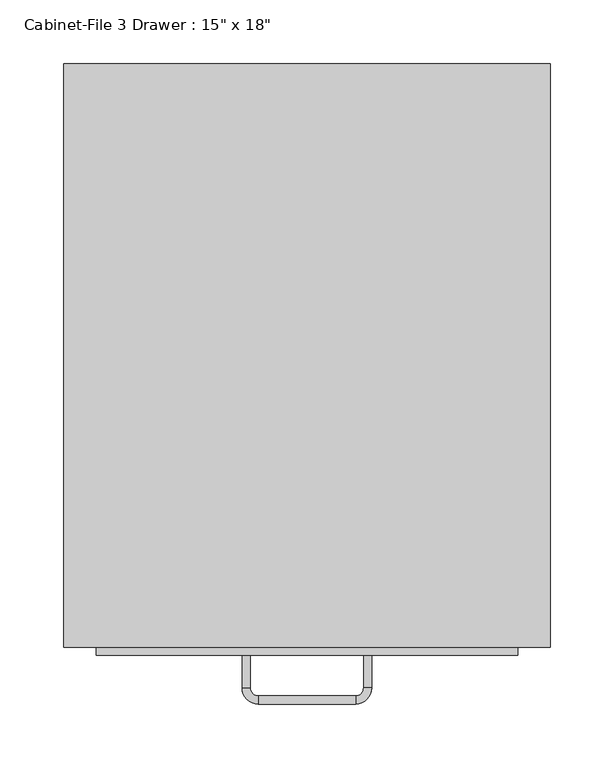
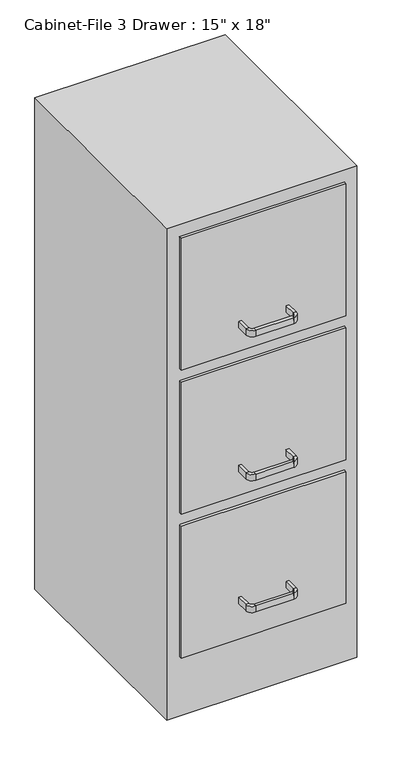
"""IFC4 building model written with IfcOpenShell, lengths in millimetres: furniture geometry."""

from ifc_helpers import new_model, si_unit, frame, origin, origin_with_axes, place, context, project, spatial, polyline, circle_curve, outline, extrude, source, transform, mapped, element, save
from ifc_brep_helpers import plane_surface, cylinder_surface, revolved_surface, advanced_brep


def furniture_552c1472(model_context):
    return source(origin(), model_context, "Body", "SolidModel", [
        extrude(outline(polyline([(62.603553, 86.4656999), (62.603553, -370.7343001), (-318.396447, -370.7343001), (-318.396447, 86.4656999), (62.603553, 86.4656999)])), origin_with_axes(), (0.0, 0.0, 1.0), 1041.4),
        extrude(outline(polyline([(37.203553, -377.0843001), (-292.996447, -377.0843001), (-292.996447, -370.7343001), (37.203553, -370.7343001), (37.203553, -377.0843001)])), frame((0.0, 0.0, 736.6), z_axis=(0.0, 0.0, 1.0), x_axis=(1.0, 0.0, 0.0)), (0.0, 0.0, 1.0), 279.4),
        extrude(outline(polyline([(37.203553, -377.0843001), (-292.996447, -377.0843001), (-292.996447, -370.7343001), (37.203553, -370.7343001), (37.203553, -377.0843001)])), frame((0.0, 0.0, 431.8), z_axis=(0.0, 0.0, 1.0), x_axis=(1.0, 0.0, 0.0)), (0.0, 0.0, 1.0), 279.4),
        extrude(outline(polyline([(37.203553, -377.0843001), (-292.996447, -377.0843001), (-292.996447, -370.7343001), (37.203553, -370.7343001), (37.203553, -377.0843001)])), frame((0.0, 0.0, 127.0), z_axis=(0.0, 0.0, 1.0), x_axis=(1.0, 0.0, 0.0)), (0.0, 0.0, 1.0), 279.4),
        advanced_brep(
        [(-172.346447, -377.0843001, 203.2), (-178.696447, -377.0843001, 203.2), (-178.696447, -377.0843001, 215.9), (-172.346447, -377.0843001, 215.9), (-172.346447, -402.4843001, 203.2), (-178.696447, -402.4843001, 203.2), (-178.696447, -402.4843001, 215.9), (-172.346447, -402.4843001, 215.9), (-165.996447, -415.1843001, 203.2), (-165.996447, -408.8343001, 203.2), (-165.996447, -415.1843001, 215.9), (-165.996447, -408.8343001, 215.9), (-89.796447, -408.8343001, 203.2), (-89.796447, -415.1843001, 203.2), (-89.796447, -415.1843001, 215.9), (-89.796447, -408.8343001, 215.9), (-77.096447, -402.4843001, 203.2), (-83.446447, -402.4843001, 203.2), (-77.096447, -402.4843001, 215.9), (-83.446447, -402.4843001, 215.9), (-83.446447, -377.0843001, 203.2), (-83.446447, -377.0843001, 215.9), (-77.096447, -377.0843001, 215.9), (-77.096447, -377.0843001, 203.2)],
        [
            (0, 1),
            (1, 2),
            (2, 3),
            (3, 0),
            (0, 4),
            (4, 5),
            (5, 1),
            (5, 6),
            (6, 2),
            (6, 7),
            (7, 3),
            (7, 4),
            (8, 5, circle_curve(frame((-165.996447, -402.4843001, 203.2), z_axis=(0.0, 0.0, -1.0), x_axis=(-1.0, 0.0, 0.0)), 12.7)),
            (4, 9, circle_curve(frame((-165.996447, -402.4843001, 203.2), z_axis=(0.0, 0.0, 1.0), x_axis=(-1.0, 0.0, 0.0)), 6.35)),
            (9, 8),
            (10, 6, circle_curve(frame((-165.996447, -402.4843001, 215.9), z_axis=(0.0, 0.0, -1.0), x_axis=(-1.0, 0.0, 0.0)), 12.7)),
            (8, 10),
            (11, 7, circle_curve(frame((-165.996447, -402.4843001, 215.9), z_axis=(0.0, 0.0, -1.0), x_axis=(-1.0, 0.0, 0.0)), 6.35)),
            (10, 11),
            (11, 9),
            (9, 12),
            (12, 13),
            (13, 8),
            (13, 14),
            (14, 10),
            (14, 15),
            (15, 11),
            (15, 12),
            (16, 13, circle_curve(frame((-89.796447, -402.4843001, 203.2), z_axis=(0.0, 0.0, -1.0), x_axis=(0.0, -1.0, 0.0)), 12.7)),
            (12, 17, circle_curve(frame((-89.796447, -402.4843001, 203.2), z_axis=(0.0, 0.0, 1.0), x_axis=(0.0, -1.0, 0.0)), 6.35)),
            (17, 16),
            (18, 14, circle_curve(frame((-89.796447, -402.4843001, 215.9), z_axis=(0.0, 0.0, -1.0), x_axis=(0.0, -1.0, 0.0)), 12.7)),
            (16, 18),
            (19, 15, circle_curve(frame((-89.796447, -402.4843001, 215.9), z_axis=(0.0, 0.0, -1.0), x_axis=(0.0, -1.0, 0.0)), 6.35)),
            (18, 19),
            (19, 17),
            (20, 21),
            (21, 22),
            (22, 23),
            (23, 20),
            (17, 20),
            (23, 16),
            (22, 18),
            (21, 19),
        ],
        [
            plane_surface(frame((-978.8216451, -377.0843001, 0.0), z_axis=(0.0, 1.0, 0.0), x_axis=(0.0, 0.0, -1.0))),
            plane_surface(frame((-172.346447, -377.0843001, 203.2), z_axis=(0.0, 0.0, -1.0), x_axis=(0.0, -1.0, 0.0))),
            plane_surface(frame((-178.696447, -377.0843001, 203.2), z_axis=(-1.0, 0.0, 0.0), x_axis=(0.0, -1.0, 0.0))),
            plane_surface(frame((-178.696447, -377.0843001, 215.9), z_axis=(0.0, 0.0, 1.0), x_axis=(0.0, -1.0, 0.0))),
            plane_surface(frame((-172.346447, -377.0843001, 215.9), z_axis=(1.0, 0.0, 0.0), x_axis=(0.0, -1.0, 0.0))),
            plane_surface(frame((-165.996447, -402.4843001, 203.2), z_axis=(0.0, 0.0, -1.0), x_axis=(-1.0, 0.0, 0.0))),
            cylinder_surface(frame((-165.996447, -402.4843001, 0.0), z_axis=(0.0, 0.0, 1.0), x_axis=(-1.0, 0.0, 0.0)), 12.7),
            plane_surface(frame((-165.996447, -402.4843001, 215.9), z_axis=(0.0, 0.0, 1.0), x_axis=(-1.0, 0.0, 0.0))),
            revolved_surface(polyline([(-172.34644699999998, -402.4843001, 215.9), (-172.34644699999998, -402.4843001, 203.2)]), (-165.996447, -402.4843001, 0.0), (0.0, 0.0, 1.0)),
            plane_surface(frame((-165.996447, -408.8343001, 203.2), z_axis=(0.0, 0.0, -1.0), x_axis=(1.0, 0.0, 0.0))),
            plane_surface(frame((-165.996447, -415.1843001, 203.2), z_axis=(0.0, -1.0, 0.0), x_axis=(1.0, 0.0, 0.0))),
            plane_surface(frame((-165.996447, -415.1843001, 215.9), z_axis=(0.0, 0.0, 1.0), x_axis=(1.0, 0.0, 0.0))),
            plane_surface(frame((-165.996447, -408.8343001, 215.9), z_axis=(0.0, 1.0, 0.0), x_axis=(1.0, 0.0, 0.0))),
            plane_surface(frame((-89.796447, -402.4843001, 203.2), z_axis=(0.0, 0.0, -1.0), x_axis=(0.0, -1.0, 0.0))),
            cylinder_surface(frame((-89.796447, -402.4843001, 0.0), z_axis=(0.0, 0.0, 1.0), x_axis=(0.0, -1.0, 0.0)), 12.7),
            plane_surface(frame((-89.796447, -402.4843001, 215.9), z_axis=(0.0, 0.0, 1.0), x_axis=(0.0, -1.0, 0.0))),
            revolved_surface(polyline([(-89.796447, -408.8343001, 215.9), (-89.796447, -408.8343001, 203.2)]), (-89.796447, -402.4843001, 0.0), (0.0, 0.0, 1.0)),
            plane_surface(frame((-877.2216451, -377.0843001, 0.0), z_axis=(0.0, 1.0, 0.0), x_axis=(0.0, 0.0, 1.0))),
            plane_surface(frame((-83.446447, -402.4843001, 203.2), z_axis=(0.0, 0.0, -1.0), x_axis=(0.0, 1.0, 0.0))),
            plane_surface(frame((-77.096447, -402.4843001, 203.2), z_axis=(1.0, 0.0, 0.0), x_axis=(0.0, 1.0, 0.0))),
            plane_surface(frame((-77.096447, -402.4843001, 215.9), z_axis=(0.0, 0.0, 1.0), x_axis=(0.0, 1.0, 0.0))),
            plane_surface(frame((-83.446447, -402.4843001, 215.9), z_axis=(-1.0, 0.0, 0.0), x_axis=(0.0, 1.0, 0.0))),
        ],
        [
            (0, [[1, 2, 3, 4]]),
            (1, [[-1, 5, 6, 7]]),
            (2, [[-2, -7, 8, 9]]),
            (3, [[-3, -9, 10, 11]]),
            (4, [[-4, -11, 12, -5]]),
            (5, [[13, -6, 14, 15]]),
            (6, [[16, -8, -13, 17]]),
            (7, [[18, -10, -16, 19]]),
            (8, [[-14, -12, -18, 20]]),
            (9, [[-15, 21, 22, 23]]),
            (10, [[-17, -23, 24, 25]]),
            (11, [[-19, -25, 26, 27]]),
            (12, [[-20, -27, 28, -21]]),
            (13, [[29, -22, 30, 31]]),
            (14, [[32, -24, -29, 33]]),
            (15, [[34, -26, -32, 35]]),
            (16, [[-30, -28, -34, 36]]),
            (17, [[37, 38, 39, 40]]),
            (18, [[-31, 41, -40, 42]]),
            (19, [[-33, -42, -39, 43]]),
            (20, [[-35, -43, -38, 44]]),
            (21, [[-36, -44, -37, -41]]),
        ],
    ),
        advanced_brep(
        [(-172.346447, -377.0843001, 482.6), (-178.696447, -377.0843001, 482.6), (-178.696447, -377.0843001, 495.3), (-172.346447, -377.0843001, 495.3), (-172.346447, -402.4843001, 482.6), (-178.696447, -402.4843001, 482.6), (-178.696447, -402.4843001, 495.3), (-172.346447, -402.4843001, 495.3), (-165.996447, -415.1843001, 482.6), (-165.996447, -408.8343001, 482.6), (-165.996447, -415.1843001, 495.3), (-165.996447, -408.8343001, 495.3), (-89.796447, -408.8343001, 482.6), (-89.796447, -415.1843001, 482.6), (-89.796447, -415.1843001, 495.3), (-89.796447, -408.8343001, 495.3), (-77.096447, -402.4843001, 482.6), (-83.446447, -402.4843001, 482.6), (-77.096447, -402.4843001, 495.3), (-83.446447, -402.4843001, 495.3), (-83.446447, -377.0843001, 482.6), (-83.446447, -377.0843001, 495.3), (-77.096447, -377.0843001, 495.3), (-77.096447, -377.0843001, 482.6)],
        [
            (0, 1),
            (1, 2),
            (2, 3),
            (3, 0),
            (0, 4),
            (4, 5),
            (5, 1),
            (5, 6),
            (6, 2),
            (6, 7),
            (7, 3),
            (7, 4),
            (8, 5, circle_curve(frame((-165.996447, -402.4843001, 482.6), z_axis=(0.0, 0.0, -1.0), x_axis=(-1.0, 0.0, 0.0)), 12.7)),
            (4, 9, circle_curve(frame((-165.996447, -402.4843001, 482.6), z_axis=(0.0, 0.0, 1.0), x_axis=(-1.0, 0.0, 0.0)), 6.35)),
            (9, 8),
            (10, 6, circle_curve(frame((-165.996447, -402.4843001, 495.3), z_axis=(0.0, 0.0, -1.0), x_axis=(-1.0, 0.0, 0.0)), 12.7)),
            (8, 10),
            (11, 7, circle_curve(frame((-165.996447, -402.4843001, 495.3), z_axis=(0.0, 0.0, -1.0), x_axis=(-1.0, 0.0, 0.0)), 6.35)),
            (10, 11),
            (11, 9),
            (9, 12),
            (12, 13),
            (13, 8),
            (13, 14),
            (14, 10),
            (14, 15),
            (15, 11),
            (15, 12),
            (16, 13, circle_curve(frame((-89.796447, -402.4843001, 482.6), z_axis=(0.0, 0.0, -1.0), x_axis=(0.0, -1.0, 0.0)), 12.7)),
            (12, 17, circle_curve(frame((-89.796447, -402.4843001, 482.6), z_axis=(0.0, 0.0, 1.0), x_axis=(0.0, -1.0, 0.0)), 6.35)),
            (17, 16),
            (18, 14, circle_curve(frame((-89.796447, -402.4843001, 495.3), z_axis=(0.0, 0.0, -1.0), x_axis=(0.0, -1.0, 0.0)), 12.7)),
            (16, 18),
            (19, 15, circle_curve(frame((-89.796447, -402.4843001, 495.3), z_axis=(0.0, 0.0, -1.0), x_axis=(0.0, -1.0, 0.0)), 6.35)),
            (18, 19),
            (19, 17),
            (20, 21),
            (21, 22),
            (22, 23),
            (23, 20),
            (17, 20),
            (23, 16),
            (22, 18),
            (21, 19),
        ],
        [
            plane_surface(frame((-978.8216451, -377.0843001, 0.0), z_axis=(0.0, 1.0, 0.0), x_axis=(0.0, 0.0, -1.0))),
            plane_surface(frame((-172.346447, -377.0843001, 482.6), z_axis=(0.0, 0.0, -1.0), x_axis=(0.0, -1.0, 0.0))),
            plane_surface(frame((-178.696447, -377.0843001, 482.6), z_axis=(-1.0, 0.0, 0.0), x_axis=(0.0, -1.0, 0.0))),
            plane_surface(frame((-178.696447, -377.0843001, 495.3), z_axis=(0.0, 0.0, 1.0), x_axis=(0.0, -1.0, 0.0))),
            plane_surface(frame((-172.346447, -377.0843001, 495.3), z_axis=(1.0, 0.0, 0.0), x_axis=(0.0, -1.0, 0.0))),
            plane_surface(frame((-165.996447, -402.4843001, 482.6), z_axis=(0.0, 0.0, -1.0), x_axis=(-1.0, 0.0, 0.0))),
            cylinder_surface(frame((-165.996447, -402.4843001, 0.0), z_axis=(0.0, 0.0, 1.0), x_axis=(-1.0, 0.0, 0.0)), 12.7),
            plane_surface(frame((-165.996447, -402.4843001, 495.3), z_axis=(0.0, 0.0, 1.0), x_axis=(-1.0, 0.0, 0.0))),
            revolved_surface(polyline([(-172.34644699999998, -402.4843001, 495.3), (-172.34644699999998, -402.4843001, 482.6)]), (-165.996447, -402.4843001, 0.0), (0.0, 0.0, 1.0)),
            plane_surface(frame((-165.996447, -408.8343001, 482.6), z_axis=(0.0, 0.0, -1.0), x_axis=(1.0, 0.0, 0.0))),
            plane_surface(frame((-165.996447, -415.1843001, 482.6), z_axis=(0.0, -1.0, 0.0), x_axis=(1.0, 0.0, 0.0))),
            plane_surface(frame((-165.996447, -415.1843001, 495.3), z_axis=(0.0, 0.0, 1.0), x_axis=(1.0, 0.0, 0.0))),
            plane_surface(frame((-165.996447, -408.8343001, 495.3), z_axis=(0.0, 1.0, 0.0), x_axis=(1.0, 0.0, 0.0))),
            plane_surface(frame((-89.796447, -402.4843001, 482.6), z_axis=(0.0, 0.0, -1.0), x_axis=(0.0, -1.0, 0.0))),
            cylinder_surface(frame((-89.796447, -402.4843001, 0.0), z_axis=(0.0, 0.0, 1.0), x_axis=(0.0, -1.0, 0.0)), 12.7),
            plane_surface(frame((-89.796447, -402.4843001, 495.3), z_axis=(0.0, 0.0, 1.0), x_axis=(0.0, -1.0, 0.0))),
            revolved_surface(polyline([(-89.796447, -408.8343001, 495.3), (-89.796447, -408.8343001, 482.6)]), (-89.796447, -402.4843001, 0.0), (0.0, 0.0, 1.0)),
            plane_surface(frame((-877.2216451, -377.0843001, 0.0), z_axis=(0.0, 1.0, 0.0), x_axis=(0.0, 0.0, 1.0))),
            plane_surface(frame((-83.446447, -402.4843001, 482.6), z_axis=(0.0, 0.0, -1.0), x_axis=(0.0, 1.0, 0.0))),
            plane_surface(frame((-77.096447, -402.4843001, 482.6), z_axis=(1.0, 0.0, 0.0), x_axis=(0.0, 1.0, 0.0))),
            plane_surface(frame((-77.096447, -402.4843001, 495.3), z_axis=(0.0, 0.0, 1.0), x_axis=(0.0, 1.0, 0.0))),
            plane_surface(frame((-83.446447, -402.4843001, 495.3), z_axis=(-1.0, 0.0, 0.0), x_axis=(0.0, 1.0, 0.0))),
        ],
        [
            (0, [[1, 2, 3, 4]]),
            (1, [[-1, 5, 6, 7]]),
            (2, [[-2, -7, 8, 9]]),
            (3, [[-3, -9, 10, 11]]),
            (4, [[-4, -11, 12, -5]]),
            (5, [[13, -6, 14, 15]]),
            (6, [[16, -8, -13, 17]]),
            (7, [[18, -10, -16, 19]]),
            (8, [[-14, -12, -18, 20]]),
            (9, [[-15, 21, 22, 23]]),
            (10, [[-17, -23, 24, 25]]),
            (11, [[-19, -25, 26, 27]]),
            (12, [[-20, -27, 28, -21]]),
            (13, [[29, -22, 30, 31]]),
            (14, [[32, -24, -29, 33]]),
            (15, [[34, -26, -32, 35]]),
            (16, [[-30, -28, -34, 36]]),
            (17, [[37, 38, 39, 40]]),
            (18, [[-31, 41, -40, 42]]),
            (19, [[-33, -42, -39, 43]]),
            (20, [[-35, -43, -38, 44]]),
            (21, [[-36, -44, -37, -41]]),
        ],
    ),
        advanced_brep(
        [(-172.346447, -377.0843001, 787.4), (-178.696447, -377.0843001, 787.4), (-178.696447, -377.0843001, 800.1), (-172.346447, -377.0843001, 800.1), (-172.346447, -402.4843001, 787.4), (-178.696447, -402.4843001, 787.4), (-178.696447, -402.4843001, 800.1), (-172.346447, -402.4843001, 800.1), (-165.996447, -415.1843001, 787.4), (-165.996447, -408.8343001, 787.4), (-165.996447, -415.1843001, 800.1), (-165.996447, -408.8343001, 800.1), (-89.796447, -408.8343001, 787.4), (-89.796447, -415.1843001, 787.4), (-89.796447, -415.1843001, 800.1), (-89.796447, -408.8343001, 800.1), (-77.096447, -402.4843001, 787.4), (-83.446447, -402.4843001, 787.4), (-77.096447, -402.4843001, 800.1), (-83.446447, -402.4843001, 800.1), (-83.446447, -377.0843001, 787.4), (-83.446447, -377.0843001, 800.1), (-77.096447, -377.0843001, 800.1), (-77.096447, -377.0843001, 787.4)],
        [
            (0, 1),
            (1, 2),
            (2, 3),
            (3, 0),
            (0, 4),
            (4, 5),
            (5, 1),
            (5, 6),
            (6, 2),
            (6, 7),
            (7, 3),
            (7, 4),
            (8, 5, circle_curve(frame((-165.996447, -402.4843001, 787.4), z_axis=(0.0, 0.0, -1.0), x_axis=(-1.0, 0.0, 0.0)), 12.7)),
            (4, 9, circle_curve(frame((-165.996447, -402.4843001, 787.4), z_axis=(0.0, 0.0, 1.0), x_axis=(-1.0, 0.0, 0.0)), 6.35)),
            (9, 8),
            (10, 6, circle_curve(frame((-165.996447, -402.4843001, 800.1), z_axis=(0.0, 0.0, -1.0), x_axis=(-1.0, 0.0, 0.0)), 12.7)),
            (8, 10),
            (11, 7, circle_curve(frame((-165.996447, -402.4843001, 800.1), z_axis=(0.0, 0.0, -1.0), x_axis=(-1.0, 0.0, 0.0)), 6.35)),
            (10, 11),
            (11, 9),
            (9, 12),
            (12, 13),
            (13, 8),
            (13, 14),
            (14, 10),
            (14, 15),
            (15, 11),
            (15, 12),
            (16, 13, circle_curve(frame((-89.796447, -402.4843001, 787.4), z_axis=(0.0, 0.0, -1.0), x_axis=(0.0, -1.0, 0.0)), 12.7)),
            (12, 17, circle_curve(frame((-89.796447, -402.4843001, 787.4), z_axis=(0.0, 0.0, 1.0), x_axis=(0.0, -1.0, 0.0)), 6.35)),
            (17, 16),
            (18, 14, circle_curve(frame((-89.796447, -402.4843001, 800.1), z_axis=(0.0, 0.0, -1.0), x_axis=(0.0, -1.0, 0.0)), 12.7)),
            (16, 18),
            (19, 15, circle_curve(frame((-89.796447, -402.4843001, 800.1), z_axis=(0.0, 0.0, -1.0), x_axis=(0.0, -1.0, 0.0)), 6.35)),
            (18, 19),
            (19, 17),
            (20, 21),
            (21, 22),
            (22, 23),
            (23, 20),
            (17, 20),
            (23, 16),
            (22, 18),
            (21, 19),
        ],
        [
            plane_surface(frame((-978.8216451, -377.0843001, 0.0), z_axis=(0.0, 1.0, 0.0), x_axis=(0.0, 0.0, -1.0))),
            plane_surface(frame((-172.346447, -377.0843001, 787.4), z_axis=(0.0, 0.0, -1.0), x_axis=(0.0, -1.0, 0.0))),
            plane_surface(frame((-178.696447, -377.0843001, 787.4), z_axis=(-1.0, 0.0, 0.0), x_axis=(0.0, -1.0, 0.0))),
            plane_surface(frame((-178.696447, -377.0843001, 800.1), z_axis=(0.0, 0.0, 1.0), x_axis=(0.0, -1.0, 0.0))),
            plane_surface(frame((-172.346447, -377.0843001, 800.1), z_axis=(1.0, 0.0, 0.0), x_axis=(0.0, -1.0, 0.0))),
            plane_surface(frame((-165.996447, -402.4843001, 787.4), z_axis=(0.0, 0.0, -1.0), x_axis=(-1.0, 0.0, 0.0))),
            cylinder_surface(frame((-165.996447, -402.4843001, 0.0), z_axis=(0.0, 0.0, 1.0), x_axis=(-1.0, 0.0, 0.0)), 12.7),
            plane_surface(frame((-165.996447, -402.4843001, 800.1), z_axis=(0.0, 0.0, 1.0), x_axis=(-1.0, 0.0, 0.0))),
            revolved_surface(polyline([(-172.34644699999998, -402.4843001, 800.1), (-172.34644699999998, -402.4843001, 787.4)]), (-165.996447, -402.4843001, 0.0), (0.0, 0.0, 1.0)),
            plane_surface(frame((-165.996447, -408.8343001, 787.4), z_axis=(0.0, 0.0, -1.0), x_axis=(1.0, 0.0, 0.0))),
            plane_surface(frame((-165.996447, -415.1843001, 787.4), z_axis=(0.0, -1.0, 0.0), x_axis=(1.0, 0.0, 0.0))),
            plane_surface(frame((-165.996447, -415.1843001, 800.1), z_axis=(0.0, 0.0, 1.0), x_axis=(1.0, 0.0, 0.0))),
            plane_surface(frame((-165.996447, -408.8343001, 800.1), z_axis=(0.0, 1.0, 0.0), x_axis=(1.0, 0.0, 0.0))),
            plane_surface(frame((-89.796447, -402.4843001, 787.4), z_axis=(0.0, 0.0, -1.0), x_axis=(0.0, -1.0, 0.0))),
            cylinder_surface(frame((-89.796447, -402.4843001, 0.0), z_axis=(0.0, 0.0, 1.0), x_axis=(0.0, -1.0, 0.0)), 12.7),
            plane_surface(frame((-89.796447, -402.4843001, 800.1), z_axis=(0.0, 0.0, 1.0), x_axis=(0.0, -1.0, 0.0))),
            revolved_surface(polyline([(-89.796447, -408.8343001, 800.1), (-89.796447, -408.8343001, 787.4)]), (-89.796447, -402.4843001, 0.0), (0.0, 0.0, 1.0)),
            plane_surface(frame((-877.2216451, -377.0843001, 0.0), z_axis=(0.0, 1.0, 0.0), x_axis=(0.0, 0.0, 1.0))),
            plane_surface(frame((-83.446447, -402.4843001, 787.4), z_axis=(0.0, 0.0, -1.0), x_axis=(0.0, 1.0, 0.0))),
            plane_surface(frame((-77.096447, -402.4843001, 787.4), z_axis=(1.0, 0.0, 0.0), x_axis=(0.0, 1.0, 0.0))),
            plane_surface(frame((-77.096447, -402.4843001, 800.1), z_axis=(0.0, 0.0, 1.0), x_axis=(0.0, 1.0, 0.0))),
            plane_surface(frame((-83.446447, -402.4843001, 800.1), z_axis=(-1.0, 0.0, 0.0), x_axis=(0.0, 1.0, 0.0))),
        ],
        [
            (0, [[1, 2, 3, 4]]),
            (1, [[-1, 5, 6, 7]]),
            (2, [[-2, -7, 8, 9]]),
            (3, [[-3, -9, 10, 11]]),
            (4, [[-4, -11, 12, -5]]),
            (5, [[13, -6, 14, 15]]),
            (6, [[16, -8, -13, 17]]),
            (7, [[18, -10, -16, 19]]),
            (8, [[-14, -12, -18, 20]]),
            (9, [[-15, 21, 22, 23]]),
            (10, [[-17, -23, 24, 25]]),
            (11, [[-19, -25, 26, 27]]),
            (12, [[-20, -27, 28, -21]]),
            (13, [[29, -22, 30, 31]]),
            (14, [[32, -24, -29, 33]]),
            (15, [[34, -26, -32, 35]]),
            (16, [[-30, -28, -34, 36]]),
            (17, [[37, 38, 39, 40]]),
            (18, [[-31, 41, -40, 42]]),
            (19, [[-33, -42, -39, 43]]),
            (20, [[-35, -43, -38, 44]]),
            (21, [[-36, -44, -37, -41]]),
        ],
    ),
    ])


if __name__ == "__main__":
    model = new_model("IFC4")
    model_context = context("Model", 3, world=origin())
    ifc_project = project(units=[si_unit("LENGTHUNIT", "METRE", prefix="MILLI")], contexts=[model_context])
    site = spatial("IfcSite", under=ifc_project)
    building = spatial("IfcBuilding", under=site)
    placement = place(None, origin())
    furniture_shape = furniture_552c1472(model_context)
    element("IfcFurniture", 1, ObjectType="Cabinet-File 3 Drawer : 15\" x 18\"", at=placement, inside=building, context=model_context, shape_type="MappedRepresentation", body=[
        mapped(furniture_shape, transform((0.0, 0.0, 0.0), x_axis=(1.0, 0.0, 0.0), y_axis=(0.0, 1.0, 0.0), z_axis=(0.0, 0.0, 1.0))),
    ])
    save(model, "model.ifc")

# Revit data of these elements
# Type "Cabinet-File 3 Drawer : 15\" x 18\""
#   Assembly Code = "E2020200"
#   Depth = 1' - 6"
#   Height = 3' - 5"
#   Width = 1' - 3"
#   Cabinet Material = Steel, Paint Finish, Ivory, Glossy
#   Handle Material = Steel, Chrome Plated
#   Default Elevation = 0
# Element 1 (IfcFurniture, "Cabinet-File 3 Drawer : 15\" x 18\"")
#   Materials on its faces: "Steel, Chrome Plated", "Steel, Paint Finish, Ivory, Glossy"
# Materials
#   "Steel, Paint Finish, Ivory, Glossy": class "Metal", colour RGB 247 247 239, transparency 0, Description = "Steel, paint finish, ivory, glossy", Cost = 0
#   "Steel, Chrome Plated": class "Metal", colour RGB 17 17 17, transparency 0, Description = "Chromiuim plated steel", Cost = 0
